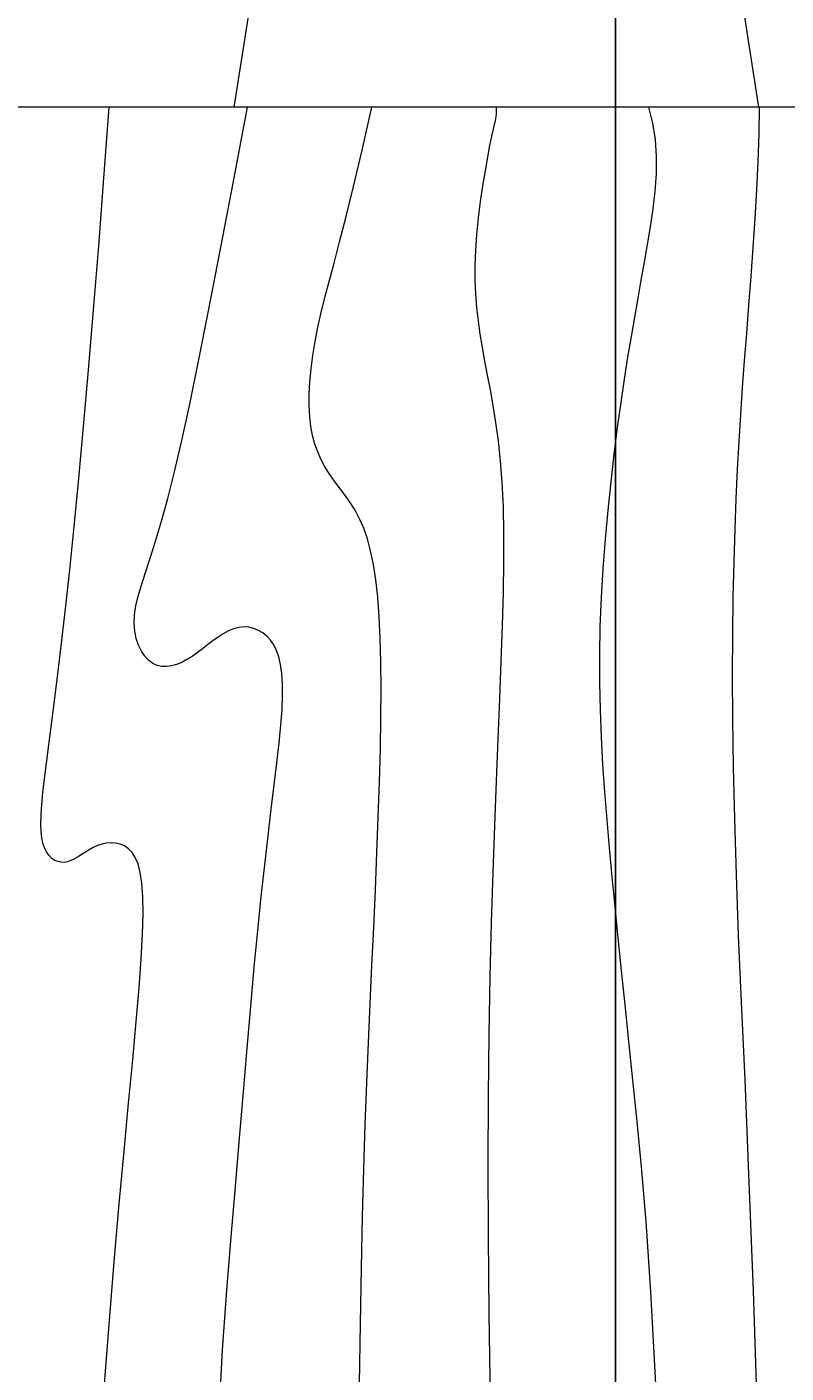
# Model space of a CAD drawing. Units: feet. Extents: x 1654 to 2985, y 1348 to 2230.
# Tile 29 of 53: x 1977 to 2002, y 1820 to 1863. Entities that reach past the tile are written whole.
import ezdxf

# ---------------------------------------------------------------- set-up
doc = ezdxf.new("R2010")
doc.units = ezdxf.units.FT
doc.layers.add('A-ANNO-DIMS', color=2, linetype='Continuous', lineweight=18)
doc.layers.add('A-FURN', color=8, linetype='Continuous', lineweight=13)
doc.styles.get("Standard").update_dxf_attribs({"font": 'arial.ttf'})
doc.dimstyles.get("Standard").update_dxf_attribs({"dimtxt": 0.18, "dimasz": 0.18, "dimexe": 0.18, "dimexo": 0.0625, "dimgap": 0.09, "dimtad": 0, "dimtih": 1, "dimtoh": 1, "dimdec": 4, "dimzin": 0, "dimdsep": 46, "dimtxsty": 'Standard', "dimcen": 0.09, "dimadec": 0, "dimazin": 0, "dimtfac": 1, "dimtdec": 4, "dimtofl": 0, "dimtmove": 0, "dimatfit": 3, "dimfxl": 1, "dimtolj": 1, "dimtzin": 0, "dimarcsym": 0})

# ---------------------------------------------------------------- blocks, each defined once
blk = doc.blocks.new('Dining Set - 36 x 72 in.')
for p, q in [((36, -18), (36, 18)), ((44.0006, 8.23428), (35.9976, 9.48474)), ((35.9976, -9.48476), (43.9993, -8.2345))]:
    blk.add_line(p, q)
for points in [[(-10.4159, 14.18652), (-7.9583, 14), (-5.6904, 13.81315), (-3.6035, 13.63021), (-1.6954, 13.45508), (0.0365, 13.29166), (1.5945, 13.14388), (2.9811, 13.01562), (4.1988, 12.9108), (5.25, 12.83333), (6.1393, 12.78613), (6.8802, 12.76823), (7.4883, 12.77767), (7.9792, 12.8125), (8.3685, 12.87077), (8.6719, 12.95052), (8.9049, 13.0498), (9.0833, 13.16666), (9.2205, 13.29899), (9.3216, 13.44401), (9.3895, 13.59879), (9.4271, 13.76041), (9.4373, 13.92594), (9.4232, 14.09245), (9.3875, 14.257), (9.3333, 14.41666), (9.2638, 14.56917), (9.1836, 14.71484), (9.0975, 14.85465), (9.0104, 14.98958), (8.9272, 15.1206), (8.8529, 15.2487), (8.7922, 15.37483), (8.75, 15.5), (8.7305, 15.62467), (8.7344, 15.74739), (8.7617, 15.86621), (8.8125, 15.97916), (8.8867, 16.08431), (8.9844, 16.17968), (9.1055, 16.26334), (9.25, 16.33333), (9.4189, 16.38802), (9.6172, 16.42708), (9.8506, 16.45052), (10.125, 16.45833), (10.4463, 16.45052), (10.8203, 16.42708), (11.2529, 16.38802), (11.75, 16.33333), (12.3184, 16.26318), (12.9694, 16.17838), (13.7151, 16.07991), (14.5677, 15.96875), (15.5395, 15.84586), (16.6426, 15.71224), (17.8893, 15.56884), (19.2917, 15.41666), (20.859, 15.25667), (22.5879, 15.08984), (24.4721, 14.91715), (26.5052, 14.73958), (28.6809, 14.5581), (30.9929, 14.3737), (33.4347, 14.18733), (36, 14)], [(-11.4399, 10.03011), (-8.877, 9.89453), (-6.7154, 9.74137), (-4.7917, 9.58333), (-2.9698, 9.43082), (-1.2246, 9.28515), (0.4415, 9.14534), (2.026, 9.01041), (3.5266, 8.87939), (4.9408, 8.7513), (6.266, 8.62516), (7.5, 8.5), (8.6411, 8.37549), (9.6914, 8.2539), (10.6538, 8.13818), (11.5312, 8.03125), (12.3267, 7.93603), (13.043, 7.85547), (13.6831, 7.79248), (14.25, 7.75), (14.7471, 7.7303), (15.1797, 7.73307), (15.5537, 7.75732), (15.875, 7.80208), (16.1494, 7.86637), (16.3828, 7.94922), (16.5811, 8.04964), (16.75, 8.16666), (16.8944, 8.29915), (17.0143, 8.44531), (17.1089, 8.60319), (17.1771, 8.77083), (17.218, 8.94629), (17.2305, 9.1276), (17.2137, 9.31282), (17.1667, 9.5), (17.0895, 9.6875), (16.987, 9.875), (16.8649, 10.0625), (16.7292, 10.25), (16.5856, 10.4375), (16.4401, 10.625), (16.2985, 10.8125), (16.1667, 11), (16.05, 11.18733), (15.9518, 11.3737), (15.8752, 11.5581), (15.8229, 11.73958), (15.798, 11.91715), (15.8034, 12.08984), (15.842, 12.25667), (15.9167, 12.41666), (16.0295, 12.56836), (16.1784, 12.70833), (16.3605, 12.83268), (16.5729, 12.9375), (16.8127, 13.01888), (17.0768, 13.07291), (17.3625, 13.0957), (17.6667, 13.08333), (17.9894, 13.03312), (18.3418, 12.94726), (18.7382, 12.82918), (19.1927, 12.68229), (19.7195, 12.51001), (20.3327, 12.31575), (21.0465, 12.10294), (21.875, 11.875), (22.8357, 11.63354), (23.959, 11.37304), (25.2786, 11.08618), (26.8282, 10.76562), (28.6414, 10.40405), (30.752, 9.99414), (33.1936, 9.52856), (36, 9)], [(-10.1112, 4.94515), (-7.9167, 4.91666), (-5.909, 4.88167), (-4.0586, 4.83984), (-2.3429, 4.79215), (-0.7396, 4.73958), (0.7739, 4.6831), (2.22, 4.6237), (3.6213, 4.56233), (5, 4.5), (6.373, 4.43782), (7.7344, 4.3776), (9.0723, 4.32129), (10.375, 4.27083), (11.6309, 4.22819), (12.8281, 4.19531), (13.9551, 4.17415), (15, 4.16666), (15.954, 4.17448), (16.819, 4.19791), (17.6001, 4.23698), (18.3021, 4.29166), (18.9299, 4.36198), (19.4883, 4.44791), (19.9823, 4.54948), (20.4167, 4.66666), (20.7969, 4.79899), (21.1302, 4.94401), (21.4245, 5.09879), (21.6875, 5.26041), (21.9271, 5.42594), (22.1511, 5.59245), (22.3672, 5.757), (22.5834, 5.91666), (22.8065, 6.06868), (23.0404, 6.21093), (23.2879, 6.34147), (23.5521, 6.45833), (23.8358, 6.55957), (24.142, 6.64323), (24.4735, 6.70735), (24.8334, 6.75), (25.2235, 6.76969), (25.642, 6.76692), (26.0858, 6.74267), (26.5521, 6.69791), (27.0379, 6.63362), (27.5404, 6.55078), (28.0565, 6.45036), (28.5834, 6.33333), (29.1242, 6.19987), (29.7071, 6.04687), (30.3661, 5.87044), (31.1354, 5.66666), (32.0493, 5.43164), (33.142, 5.16146), (34.4475, 4.85221), (36, 4.5)], [(-10.6523, 0.21289), (-7.5796, 0.26522), (-4.75, 0.29166), (-2.134, 0.29793), (0.2878, 0.28711), (2.5317, 0.26163), (4.6146, 0.22396), (6.5529, 0.17651), (8.3633, 0.12174), (10.0623, 0.06209), (11.6667, 0), (13.1899, -0.06201), (14.6341, -0.1211), (15.9982, -0.17432), (17.2813, -0.21875), (18.4823, -0.25147), (19.6003, -0.26953), (20.6343, -0.27002), (21.5834, -0.25), (22.4481, -0.20768), (23.2357, -0.14584), (23.9549, -0.06836), (24.6146, 0.02083), (25.2235, 0.11784), (25.7904, 0.21875), (26.3241, 0.31966), (26.8334, 0.41666), (27.3265, 0.50618), (27.8099, 0.58593), (28.2894, 0.65397), (28.7709, 0.70833), (29.2601, 0.74707), (29.763, 0.76823), (30.2855, 0.76985), (30.8334, 0.75), (31.4088, 0.70784), (31.9994, 0.64713), (32.589, 0.57275), (33.1615, 0.48958), (33.7008, 0.4025), (34.1908, 0.3164), (34.6153, 0.23616), (34.9584, 0.16666), (35.2099, 0.11165), (35.3848, 0.07031), (35.504, 0.04069), (35.5886, 0.02083), (35.6594, 0.00879), (35.7377, 0.0026), (35.8442, 0.00032), (36, 0)], [(-10.1094, -5.76042), (-6.7752, -5.58285), (-4.2363, -5.41016), (-2.2629, -5.24333), (-0.625, -5.08334), (0.8708, -4.93099), (2.2715, -4.78646), (3.5872, -4.64974), (4.8281, -4.52084), (6.0046, -4.39974), (7.127, -4.28646), (8.2053, -4.18099), (9.25, -4.08334), (10.2705, -3.99382), (11.2734, -3.91407), (12.2647, -3.84603), (13.25, -3.79167), (14.2354, -3.75293), (15.2266, -3.73177), (16.2295, -3.73015), (17.25, -3.75), (18.2912, -3.79248), (19.3451, -3.85547), (20.4009, -3.93604), (21.4479, -4.03125), (22.4754, -4.13819), (23.4727, -4.25391), (24.4289, -4.37549), (25.3334, -4.5), (26.1785, -4.62492), (26.9694, -4.74935), (27.7145, -4.87281), (28.4219, -4.99479), (29.1, -5.11483), (29.7572, -5.23242), (30.4016, -5.34709), (31.0417, -5.45834), (31.6837, -5.56437), (32.3262, -5.65821), (32.9658, -5.73153), (33.599, -5.77604), (34.2224, -5.78345), (34.8327, -5.74545), (35.4264, -5.65373), (36, -5.5)], [(-11.9839, -9.45069), (-6.7396, -9.28125), (-2.5226, -9.12354), (0.8789, -8.98047), (3.6769, -8.85498), (6.0833, -8.75), (8.2767, -8.66765), (10.3021, -8.60677), (12.1712, -8.56543), (13.8958, -8.54167), (15.4876, -8.53353), (16.9583, -8.53907), (18.3197, -8.55632), (19.5834, -8.58334), (20.7616, -8.61841), (21.8685, -8.66081), (22.9188, -8.71004), (23.9271, -8.76563), (24.9081, -8.82707), (25.8763, -8.89388), (26.8465, -8.96558), (27.8334, -9.04167), (28.8474, -9.12118), (29.8828, -9.20117), (30.93, -9.27824), (31.9792, -9.34896), (33.0205, -9.40991), (34.0443, -9.45768), (35.0407, -9.48885), (36, -9.5)]]:
    blk.add_lwpolyline(points)
blk = doc.blocks.new('*D101')
at = {"layer": 'A-ANNO-DIMS', "color": 0, "lineweight": -2, "transparency": 16777216}
for p, q in [((1996.092, 2039.192), (1996.092, 1534.075)), ((2014.016, 2039.192), (2014.016, 1534.075)), ((1996.272, 1534.255), (2004.599, 1534.255)), ((2013.836, 1534.255), (2005.509, 1534.255))]:
    blk.add_line(p, q, dxfattribs=at)
at = {"layer": 'A-ANNO-DIMS', "color": 0, "transparency": 16777216}
for points in [[(1996.272, 1534.285), (1996.272, 1534.225), (1996.092, 1534.255)], [(2013.836, 1534.285), (2013.836, 1534.225), (2014.016, 1534.255)]]:
    blk.add_solid(points, dxfattribs=at)
at = {"layer": 'Defpoints', "color": 0, "transparency": 16777216}
for p in [(1996.092, 2039.255), (2014.016, 2039.255), (2014.016, 1534.255)]:
    blk.add_point(p, dxfattribs=at)
at = {"layer": 'A-ANNO-DIMS', "color": 0, "transparency": 16777216, "insert": (2005.054, 1534.255), "char_height": 0.18, "attachment_point": 5}
blk.add_mtext('\\A1;17.924', dxfattribs=at)

msp = doc.modelspace()

# ---------------------------------------------------------------- block references
at = {"layer": 'A-FURN', "xscale": 0.8893748792417884, "yscale": 0.8893748792417884, "zscale": 0.8893748792417884, "rotation": 90}
msp.add_blockref('Dining Set - 36 x 72 in.', (1992.2681, 1828.3522), dxfattribs=at)

# ---------------------------------------------------------------- dimensions: what is measured, and where the dimension line sits
at = {"layer": 'A-ANNO-DIMS'}
dim = msp.add_linear_dim(base=(2014.016, 1534.2549), p1=(1996.0924, 2039.2549), p2=(2014.016, 2039.2549), dimstyle='Standard', override={"dimdec": 3, "dimlfac": 1, "dimrnd": 0, "dimzin": 0, "dimdsep": 46, "dimlunit": 2}, dxfattribs=at)
dim.commit()
dim.dimension.update_dxf_attribs({"geometry": '*D101', "text_midpoint": (2005.0542, 1534.2549)})

doc.saveas('drawing.dxf')
